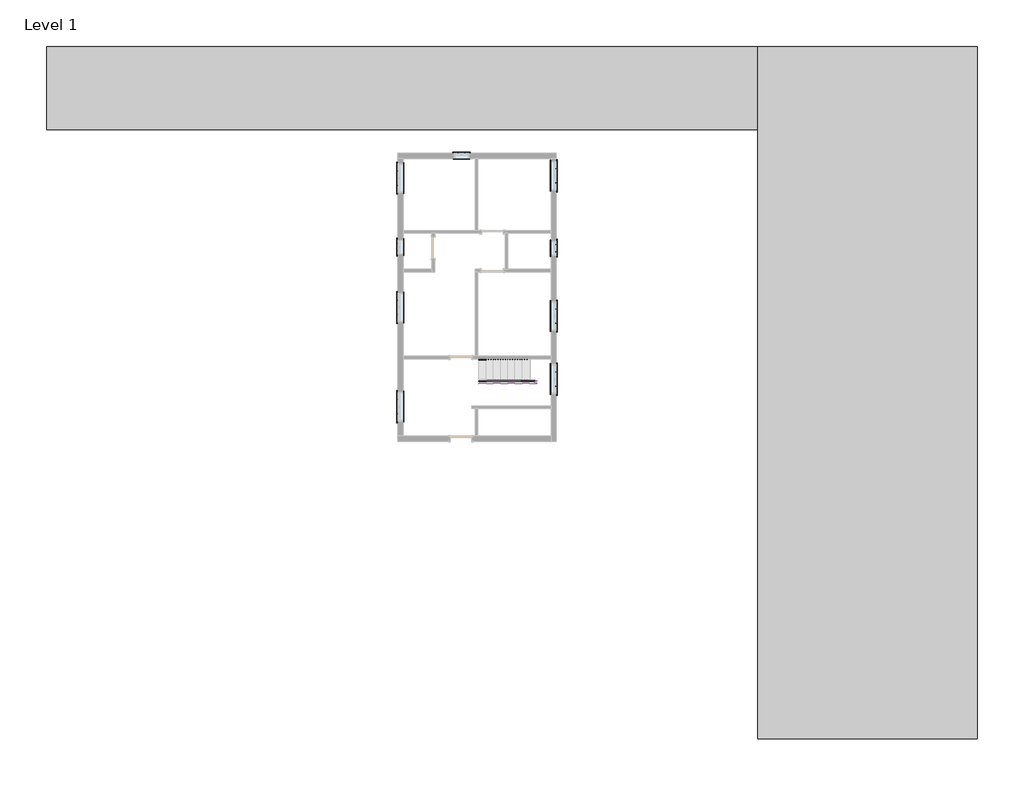
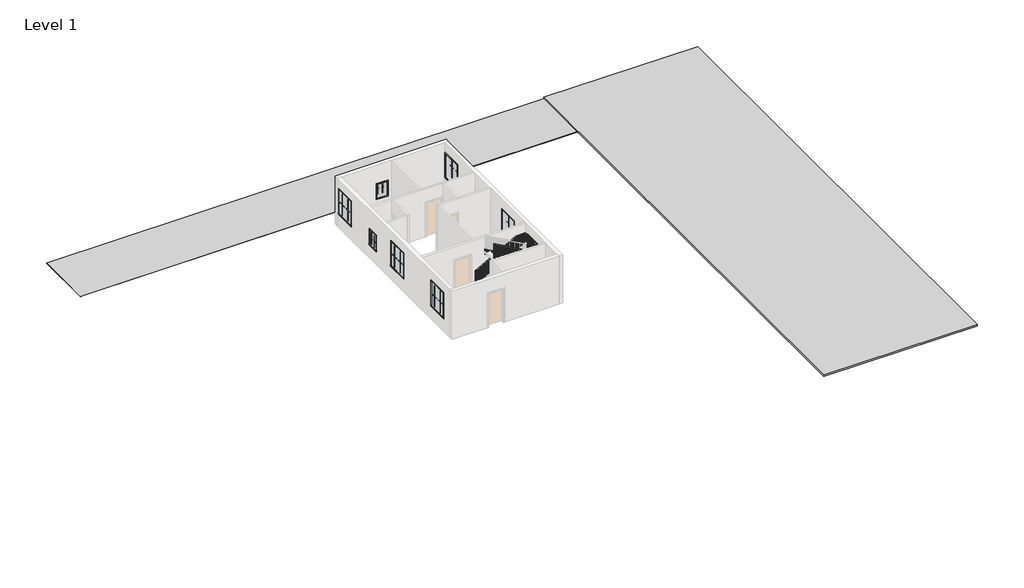
# One storey, part 2 of 2: 37 proxies, 3 members, 1 railing.
"""IFC4 building model written with IfcOpenShell, lengths in millimetres."""

from ifc_helpers import new_model, si_unit, frame, origin, place, context, project, spatial, polyline, outline, extrude, faceted_brep, transform, mapped, element, save
from components import generic_models_1_generic_models_1_c6e5ea94, muntin_pattern_2x2_muntin_pattern_2x2_6dad3731, muntin_pattern_2x2_muntin_pattern_2x2_a30a3345, muntin_pattern_2x2_muntin_pattern_2x2_53152e2c, muntin_pattern_2x2_muntin_pattern_2x2_e8f3e573, trim_window_exterior_flat_with_sill_92b9b949, trim_window_exterior_flat_with_sill_a665a915, trim_window_interior_flat_picture_frame_3bb882cf, trim_window_interior_flat_picture_frame_d485c387

model = new_model("IFC4")

# Units and contexts
model_context = context("Model", 3, world=origin())
ifc_project = project(units=[si_unit("LENGTHUNIT", "METRE", prefix="MILLI")], contexts=[model_context])

# Site, building, storey
site = spatial("IfcSite", under=ifc_project)
building = spatial("IfcBuilding", under=site)
storey = spatial("IfcBuildingStorey", under=building, Name="Level 1", Elevation=0.0)

# Proxies
placement = place(None, origin())
generic_models_1_generic_models_1_shape = generic_models_1_generic_models_1_c6e5ea94(model_context)
element("IfcBuildingElementProxy", 1, Name="Generic Models 1 : Generic Models 1", ObjectType="Generic Models 1 : Generic Models 1", at=placement, inside=storey, context=model_context, shape_type="MappedRepresentation", body=[
    mapped(generic_models_1_generic_models_1_shape, transform((0.0, 0.0, 0.0), x_axis=(1.0, 0.0, 0.0), y_axis=(0.0, 1.0, 0.0), z_axis=(0.0, 0.0, 1.0))),
])
muntin_pattern_2x2_muntin_pattern_2x2_shape = muntin_pattern_2x2_muntin_pattern_2x2_6dad3731(model_context)
element("IfcBuildingElementProxy", 2, Name="Muntin Pattern_2x2 : Muntin Pattern_2x2", ObjectType="Muntin Pattern_2x2 : Muntin Pattern_2x2", at=placement, inside=storey, context=model_context, shape_type="MappedRepresentation", body=[
    mapped(muntin_pattern_2x2_muntin_pattern_2x2_shape, transform((1279.525, 2947.4914062, 984.25), x_axis=(0.0, 1.0, 0.0), y_axis=(-1.0, 0.0, 0.0), z_axis=(0.0, 0.0, 1.0))),
])
element("IfcBuildingElementProxy", 3, Name="Muntin Pattern_2x2 : Muntin Pattern_2x2", ObjectType="Muntin Pattern_2x2 : Muntin Pattern_2x2", at=placement, inside=storey, context=model_context, shape_type="MappedRepresentation", body=[
    mapped(muntin_pattern_2x2_muntin_pattern_2x2_shape, transform((1279.525, 7141.6664062, 984.25), x_axis=(0.0, 1.0, 0.0), y_axis=(-1.0, 0.0, 0.0), z_axis=(0.0, 0.0, 1.0))),
])
element("IfcBuildingElementProxy", 4, Name="Muntin Pattern_2x2 : Muntin Pattern_2x2", ObjectType="Muntin Pattern_2x2 : Muntin Pattern_2x2", at=placement, inside=storey, context=model_context, shape_type="MappedRepresentation", body=[
    mapped(muntin_pattern_2x2_muntin_pattern_2x2_shape, transform((1279.525, 12605.8414062, 984.25), x_axis=(0.0, 1.0, 0.0), y_axis=(-1.0, 0.0, 0.0), z_axis=(0.0, 0.0, 1.0))),
])
element("IfcBuildingElementProxy", 5, Name="Muntin Pattern_2x2 : Muntin Pattern_2x2", ObjectType="Muntin Pattern_2x2 : Muntin Pattern_2x2", at=placement, inside=storey, context=model_context, shape_type="MappedRepresentation", body=[
    mapped(muntin_pattern_2x2_muntin_pattern_2x2_shape, transform((7966.075, 13308.0125, 984.25), x_axis=(0.0, -1.0, 0.0), y_axis=(1.0, 0.0, 0.0), z_axis=(0.0, 0.0, 1.0))),
])
element("IfcBuildingElementProxy", 6, Name="Muntin Pattern_2x2 : Muntin Pattern_2x2", ObjectType="Muntin Pattern_2x2 : Muntin Pattern_2x2", at=placement, inside=storey, context=model_context, shape_type="MappedRepresentation", body=[
    mapped(muntin_pattern_2x2_muntin_pattern_2x2_shape, transform((7966.075, 7377.1125, 984.25), x_axis=(0.0, -1.0, 0.0), y_axis=(1.0, 0.0, 0.0), z_axis=(0.0, 0.0, 1.0))),
])
element("IfcBuildingElementProxy", 7, Name="Muntin Pattern_2x2 : Muntin Pattern_2x2", ObjectType="Muntin Pattern_2x2 : Muntin Pattern_2x2", at=placement, inside=storey, context=model_context, shape_type="MappedRepresentation", body=[
    mapped(muntin_pattern_2x2_muntin_pattern_2x2_shape, transform((7966.075, 4716.4625, 984.25), x_axis=(0.0, -1.0, 0.0), y_axis=(1.0, 0.0, 0.0), z_axis=(0.0, 0.0, 1.0))),
])
muntin_pattern_2x2_muntin_pattern_2x2_2_shape = muntin_pattern_2x2_muntin_pattern_2x2_a30a3345(model_context)
element("IfcBuildingElementProxy", 8, Name="Muntin Pattern_2x2 : Muntin Pattern_2x2", ObjectType="Muntin Pattern_2x2 : Muntin Pattern_2x2", at=placement, inside=storey, context=model_context, shape_type="MappedRepresentation", body=[
    mapped(muntin_pattern_2x2_muntin_pattern_2x2_2_shape, transform((1279.525, 3553.9164063, 984.25), x_axis=(0.0, -1.0, 0.0), y_axis=(1.0, 0.0, 0.0), z_axis=(0.0, 0.0, 1.0))),
])
element("IfcBuildingElementProxy", 9, Name="Muntin Pattern_2x2 : Muntin Pattern_2x2", ObjectType="Muntin Pattern_2x2 : Muntin Pattern_2x2", at=placement, inside=storey, context=model_context, shape_type="MappedRepresentation", body=[
    mapped(muntin_pattern_2x2_muntin_pattern_2x2_2_shape, transform((1279.525, 7748.0914062, 984.25), x_axis=(0.0, -1.0, 0.0), y_axis=(1.0, 0.0, 0.0), z_axis=(0.0, 0.0, 1.0))),
])
element("IfcBuildingElementProxy", 10, Name="Muntin Pattern_2x2 : Muntin Pattern_2x2", ObjectType="Muntin Pattern_2x2 : Muntin Pattern_2x2", at=placement, inside=storey, context=model_context, shape_type="MappedRepresentation", body=[
    mapped(muntin_pattern_2x2_muntin_pattern_2x2_2_shape, transform((1279.525, 13212.2664062, 984.25), x_axis=(0.0, -1.0, 0.0), y_axis=(1.0, 0.0, 0.0), z_axis=(0.0, 0.0, 1.0))),
])
element("IfcBuildingElementProxy", 11, Name="Muntin Pattern_2x2 : Muntin Pattern_2x2", ObjectType="Muntin Pattern_2x2 : Muntin Pattern_2x2", at=placement, inside=storey, context=model_context, shape_type="MappedRepresentation", body=[
    mapped(muntin_pattern_2x2_muntin_pattern_2x2_2_shape, transform((7966.075, 12701.5875, 984.25), x_axis=(0.0, 1.0, 0.0), y_axis=(-1.0, 0.0, 0.0), z_axis=(0.0, 0.0, 1.0))),
])
element("IfcBuildingElementProxy", 12, Name="Muntin Pattern_2x2 : Muntin Pattern_2x2", ObjectType="Muntin Pattern_2x2 : Muntin Pattern_2x2", at=placement, inside=storey, context=model_context, shape_type="MappedRepresentation", body=[
    mapped(muntin_pattern_2x2_muntin_pattern_2x2_2_shape, transform((7966.075, 6770.6875, 984.25), x_axis=(0.0, 1.0, 0.0), y_axis=(-1.0, 0.0, 0.0), z_axis=(0.0, 0.0, 1.0))),
])
element("IfcBuildingElementProxy", 13, Name="Muntin Pattern_2x2 : Muntin Pattern_2x2", ObjectType="Muntin Pattern_2x2 : Muntin Pattern_2x2", at=placement, inside=storey, context=model_context, shape_type="MappedRepresentation", body=[
    mapped(muntin_pattern_2x2_muntin_pattern_2x2_2_shape, transform((7966.075, 4110.0375, 984.25), x_axis=(0.0, 1.0, 0.0), y_axis=(-1.0, 0.0, 0.0), z_axis=(0.0, 0.0, 1.0))),
])
muntin_pattern_2x2_muntin_pattern_2x2_3_shape = muntin_pattern_2x2_muntin_pattern_2x2_53152e2c(model_context)
element("IfcBuildingElementProxy", 14, Name="Muntin Pattern_2x2 : Muntin Pattern_2x2", ObjectType="Muntin Pattern_2x2 : Muntin Pattern_2x2", at=placement, inside=storey, context=model_context, shape_type="MappedRepresentation", body=[
    mapped(muntin_pattern_2x2_muntin_pattern_2x2_3_shape, transform((3811.5875, 13960.475, 984.25), x_axis=(1.0, 0.0, 0.0), y_axis=(0.0, 1.0, 0.0), z_axis=(0.0, 0.0, 1.0))),
])
element("IfcBuildingElementProxy", 15, Name="Muntin Pattern_2x2 : Muntin Pattern_2x2", ObjectType="Muntin Pattern_2x2 : Muntin Pattern_2x2", at=placement, inside=storey, context=model_context, shape_type="MappedRepresentation", body=[
    mapped(muntin_pattern_2x2_muntin_pattern_2x2_3_shape, transform((7966.075, 10101.2625, 984.25), x_axis=(0.0, -1.0, 0.0), y_axis=(1.0, 0.0, 0.0), z_axis=(0.0, 0.0, 1.0))),
])
element("IfcBuildingElementProxy", 16, Name="Muntin Pattern_2x2 : Muntin Pattern_2x2", ObjectType="Muntin Pattern_2x2 : Muntin Pattern_2x2", at=placement, inside=storey, context=model_context, shape_type="MappedRepresentation", body=[
    mapped(muntin_pattern_2x2_muntin_pattern_2x2_3_shape, transform((1279.525, 9843.5914062, 984.25), x_axis=(0.0, 1.0, 0.0), y_axis=(-1.0, 0.0, 0.0), z_axis=(0.0, 0.0, 1.0))),
])
muntin_pattern_2x2_muntin_pattern_2x2_4_shape = muntin_pattern_2x2_muntin_pattern_2x2_e8f3e573(model_context)
element("IfcBuildingElementProxy", 17, Name="Muntin Pattern_2x2 : Muntin Pattern_2x2", ObjectType="Muntin Pattern_2x2 : Muntin Pattern_2x2", at=placement, inside=storey, context=model_context, shape_type="MappedRepresentation", body=[
    mapped(muntin_pattern_2x2_muntin_pattern_2x2_4_shape, transform((4113.2125, 13960.475, 984.25), x_axis=(-1.0, 0.0, 0.0), y_axis=(0.0, -1.0, 0.0), z_axis=(0.0, 0.0, 1.0))),
])
element("IfcBuildingElementProxy", 18, Name="Muntin Pattern_2x2 : Muntin Pattern_2x2", ObjectType="Muntin Pattern_2x2 : Muntin Pattern_2x2", at=placement, inside=storey, context=model_context, shape_type="MappedRepresentation", body=[
    mapped(muntin_pattern_2x2_muntin_pattern_2x2_4_shape, transform((7966.075, 9799.6375, 984.25), x_axis=(0.0, 1.0, 0.0), y_axis=(-1.0, 0.0, 0.0), z_axis=(0.0, 0.0, 1.0))),
])
element("IfcBuildingElementProxy", 19, Name="Muntin Pattern_2x2 : Muntin Pattern_2x2", ObjectType="Muntin Pattern_2x2 : Muntin Pattern_2x2", at=placement, inside=storey, context=model_context, shape_type="MappedRepresentation", body=[
    mapped(muntin_pattern_2x2_muntin_pattern_2x2_4_shape, transform((1279.525, 10145.2164062, 984.25), x_axis=(0.0, -1.0, 0.0), y_axis=(1.0, 0.0, 0.0), z_axis=(0.0, 0.0, 1.0))),
])
trim_window_exterior_flat_with_sill_shape = trim_window_exterior_flat_with_sill_92b9b949(model_context)
element("IfcBuildingElementProxy", 20, Name="Trim-Window-Exterior-Flat : with Sill", ObjectType="Trim-Window-Exterior-Flat : with Sill", at=placement, inside=storey, context=model_context, shape_type="MappedRepresentation", body=[
    mapped(trim_window_exterior_flat_with_sill_shape, transform((1270.0, 3250.7039063, 2438.4), x_axis=(0.0, -1.0, 0.0), y_axis=(0.0, 0.0, 1.0), z_axis=(-1.0, 0.0, 0.0))),
])
element("IfcBuildingElementProxy", 21, Name="Trim-Window-Exterior-Flat : with Sill", ObjectType="Trim-Window-Exterior-Flat : with Sill", at=placement, inside=storey, context=model_context, shape_type="MappedRepresentation", body=[
    mapped(trim_window_exterior_flat_with_sill_shape, transform((1270.0, 7444.8789063, 2438.4), x_axis=(0.0, -1.0, 0.0), y_axis=(0.0, 0.0, 1.0), z_axis=(-1.0, 0.0, 0.0))),
])
element("IfcBuildingElementProxy", 22, Name="Trim-Window-Exterior-Flat : with Sill", ObjectType="Trim-Window-Exterior-Flat : with Sill", at=placement, inside=storey, context=model_context, shape_type="MappedRepresentation", body=[
    mapped(trim_window_exterior_flat_with_sill_shape, transform((1270.0, 12909.0539063, 2438.4), x_axis=(0.0, -1.0, 0.0), y_axis=(0.0, 0.0, 1.0), z_axis=(-1.0, 0.0, 0.0))),
])
element("IfcBuildingElementProxy", 23, Name="Trim-Window-Exterior-Flat : with Sill", ObjectType="Trim-Window-Exterior-Flat : with Sill", at=placement, inside=storey, context=model_context, shape_type="MappedRepresentation", body=[
    mapped(trim_window_exterior_flat_with_sill_shape, transform((7975.6, 13004.8, 2438.4), x_axis=(0.0, 1.0, 0.0), y_axis=(0.0, 0.0, 1.0), z_axis=(1.0, 0.0, 0.0))),
])
element("IfcBuildingElementProxy", 24, Name="Trim-Window-Exterior-Flat : with Sill", ObjectType="Trim-Window-Exterior-Flat : with Sill", at=placement, inside=storey, context=model_context, shape_type="MappedRepresentation", body=[
    mapped(trim_window_exterior_flat_with_sill_shape, transform((7975.6, 7073.9, 2438.4), x_axis=(0.0, 1.0, 0.0), y_axis=(0.0, 0.0, 1.0), z_axis=(1.0, 0.0, 0.0))),
])
element("IfcBuildingElementProxy", 25, Name="Trim-Window-Exterior-Flat : with Sill", ObjectType="Trim-Window-Exterior-Flat : with Sill", at=placement, inside=storey, context=model_context, shape_type="MappedRepresentation", body=[
    mapped(trim_window_exterior_flat_with_sill_shape, transform((7975.6, 4413.25, 2438.4), x_axis=(0.0, 1.0, 0.0), y_axis=(0.0, 0.0, 1.0), z_axis=(1.0, 0.0, 0.0))),
])
trim_window_exterior_flat_with_sill_2_shape = trim_window_exterior_flat_with_sill_a665a915(model_context)
element("IfcBuildingElementProxy", 26, Name="Trim-Window-Exterior-Flat : with Sill", ObjectType="Trim-Window-Exterior-Flat : with Sill", at=placement, inside=storey, context=model_context, shape_type="MappedRepresentation", body=[
    mapped(trim_window_exterior_flat_with_sill_2_shape, transform((3962.4, 13970.0, 1828.8), x_axis=(-1.0, 0.0, 0.0), y_axis=(0.0, 0.0, 1.0), z_axis=(0.0, 1.0, 0.0))),
])
element("IfcBuildingElementProxy", 27, Name="Trim-Window-Exterior-Flat : with Sill", ObjectType="Trim-Window-Exterior-Flat : with Sill", at=placement, inside=storey, context=model_context, shape_type="MappedRepresentation", body=[
    mapped(trim_window_exterior_flat_with_sill_2_shape, transform((7975.6, 9950.45, 1828.8), x_axis=(0.0, 1.0, 0.0), y_axis=(0.0, 0.0, 1.0), z_axis=(1.0, 0.0, 0.0))),
])
element("IfcBuildingElementProxy", 28, Name="Trim-Window-Exterior-Flat : with Sill", ObjectType="Trim-Window-Exterior-Flat : with Sill", at=placement, inside=storey, context=model_context, shape_type="MappedRepresentation", body=[
    mapped(trim_window_exterior_flat_with_sill_2_shape, transform((1270.0, 9994.4039062, 1828.8), x_axis=(0.0, -1.0, 0.0), y_axis=(0.0, 0.0, 1.0), z_axis=(-1.0, 0.0, 0.0))),
])
trim_window_interior_flat_picture_frame_shape = trim_window_interior_flat_picture_frame_3bb882cf(model_context)
element("IfcBuildingElementProxy", 29, Name="Trim-Window-Interior-Flat : Picture Frame", ObjectType="Trim-Window-Interior-Flat : Picture Frame", at=placement, inside=storey, context=model_context, shape_type="MappedRepresentation", body=[
    mapped(trim_window_interior_flat_picture_frame_shape, transform((1498.6, 3250.7039063, 2438.4), x_axis=(0.0, 1.0, 0.0), y_axis=(0.0, 0.0, 1.0), z_axis=(1.0, 0.0, 0.0))),
])
element("IfcBuildingElementProxy", 30, Name="Trim-Window-Interior-Flat : Picture Frame", ObjectType="Trim-Window-Interior-Flat : Picture Frame", at=placement, inside=storey, context=model_context, shape_type="MappedRepresentation", body=[
    mapped(trim_window_interior_flat_picture_frame_shape, transform((1498.6, 7444.8789062, 2438.4), x_axis=(0.0, 1.0, 0.0), y_axis=(0.0, 0.0, 1.0), z_axis=(1.0, 0.0, 0.0))),
])
element("IfcBuildingElementProxy", 31, Name="Trim-Window-Interior-Flat : Picture Frame", ObjectType="Trim-Window-Interior-Flat : Picture Frame", at=placement, inside=storey, context=model_context, shape_type="MappedRepresentation", body=[
    mapped(trim_window_interior_flat_picture_frame_shape, transform((1498.6, 12909.0539062, 2438.4), x_axis=(0.0, 1.0, 0.0), y_axis=(0.0, 0.0, 1.0), z_axis=(1.0, 0.0, 0.0))),
])
element("IfcBuildingElementProxy", 32, Name="Trim-Window-Interior-Flat : Picture Frame", ObjectType="Trim-Window-Interior-Flat : Picture Frame", at=placement, inside=storey, context=model_context, shape_type="MappedRepresentation", body=[
    mapped(trim_window_interior_flat_picture_frame_shape, transform((7747.0, 13004.8, 2438.4), x_axis=(0.0, -1.0, 0.0), y_axis=(0.0, 0.0, 1.0), z_axis=(-1.0, 0.0, 0.0))),
])
element("IfcBuildingElementProxy", 33, Name="Trim-Window-Interior-Flat : Picture Frame", ObjectType="Trim-Window-Interior-Flat : Picture Frame", at=placement, inside=storey, context=model_context, shape_type="MappedRepresentation", body=[
    mapped(trim_window_interior_flat_picture_frame_shape, transform((7747.0, 7073.9, 2438.4), x_axis=(0.0, -1.0, 0.0), y_axis=(0.0, 0.0, 1.0), z_axis=(-1.0, 0.0, 0.0))),
])
element("IfcBuildingElementProxy", 34, Name="Trim-Window-Interior-Flat : Picture Frame", ObjectType="Trim-Window-Interior-Flat : Picture Frame", at=placement, inside=storey, context=model_context, shape_type="MappedRepresentation", body=[
    mapped(trim_window_interior_flat_picture_frame_shape, transform((7747.0, 4413.25, 2438.4), x_axis=(0.0, -1.0, 0.0), y_axis=(0.0, 0.0, 1.0), z_axis=(-1.0, 0.0, 0.0))),
])
trim_window_interior_flat_picture_frame_2_shape = trim_window_interior_flat_picture_frame_d485c387(model_context)
element("IfcBuildingElementProxy", 35, Name="Trim-Window-Interior-Flat : Picture Frame", ObjectType="Trim-Window-Interior-Flat : Picture Frame", at=placement, inside=storey, context=model_context, shape_type="MappedRepresentation", body=[
    mapped(trim_window_interior_flat_picture_frame_2_shape, transform((3962.4, 13741.4, 1828.8), x_axis=(1.0, 0.0, 0.0), y_axis=(0.0, 0.0, 1.0), z_axis=(0.0, -1.0, 0.0))),
])
element("IfcBuildingElementProxy", 36, Name="Trim-Window-Interior-Flat : Picture Frame", ObjectType="Trim-Window-Interior-Flat : Picture Frame", at=placement, inside=storey, context=model_context, shape_type="MappedRepresentation", body=[
    mapped(trim_window_interior_flat_picture_frame_2_shape, transform((7747.0, 9950.45, 1828.8), x_axis=(0.0, -1.0, 0.0), y_axis=(0.0, 0.0, 1.0), z_axis=(-1.0, 0.0, 0.0))),
])
element("IfcBuildingElementProxy", 37, Name="Trim-Window-Interior-Flat : Picture Frame", ObjectType="Trim-Window-Interior-Flat : Picture Frame", at=placement, inside=storey, context=model_context, shape_type="MappedRepresentation", body=[
    mapped(trim_window_interior_flat_picture_frame_2_shape, transform((1498.6, 9994.4039062, 1828.8), x_axis=(0.0, 1.0, 0.0), y_axis=(0.0, 0.0, 1.0), z_axis=(1.0, 0.0, 0.0))),
])

# Members
element("IfcMember", 38, ObjectType="Stringer - 2\" Width", at=placement, inside=storey, context=model_context, shape_type="SweptSolid", body=[
    extrude(outline(polyline([(207.5983948, 4699.0), (0.0, 4699.0), (0.0, 4952.9445028), (1185.3641651, 7086.6), (1534.0428392, 7086.6), (207.5983948, 4699.0)])), frame((0.0, 4305.3, 0.0), z_axis=(0.0, 1.0, 0.0), x_axis=(0.0, 0.0, 1.0)), (0.0, 0.0, 1.0), 50.8),
])
element("IfcMember", 39, ObjectType="Stringer - 2\" Width", at=placement, inside=storey, context=model_context, shape_type="SweptSolid", body=[
    extrude(outline(polyline([(7086.6, 4356.1), (7137.4, 4356.1), (7137.4, 4254.5), (7086.6, 4254.5), (7086.6, 4356.1)])), frame((0.0, 0.0, 1295.4), z_axis=(0.0, 0.0, 1.0), x_axis=(1.0, 0.0, 0.0)), (0.0, 0.0, 1.0), 304.8),
])
element("IfcMember", 40, ObjectType="Stringer - 2\" Width", at=placement, inside=storey, context=model_context, shape_type="SweptSolid", body=[
    extrude(outline(polyline([(1382.9197207, 7137.4), (1731.5983948, 7137.4), (3086.2650614, 4699.0), (2737.5863873, 4699.0), (1382.9197207, 7137.4)])), frame((0.0, 4203.7, 0.0), z_axis=(0.0, 1.0, 0.0), x_axis=(0.0, 0.0, 1.0)), (0.0, 0.0, 1.0), 50.8),
])

# Railing
element("IfcRailing", 41, ObjectType="Handrail - Rectangular", at=placement, inside=storey, context=model_context, shape_type="SolidModel", body=[
    faceted_brep([(4699.0, 5270.5, 1083.7333333), (4699.0, 5270.5, 1025.620221), (4699.0, 5219.7, 1025.620221), (4699.0, 5219.7, 1083.7333333), (7137.4, 5270.5, 2438.4), (7150.5636022, 5270.5, 2387.6), (7150.5636022, 5219.7, 2387.6), (7137.4, 5219.7, 2438.4), (7747.0, 5270.5, 2438.4), (7747.0, 5270.5, 2387.6), (7696.2, 5219.7, 2387.6), (7696.2, 5219.7, 2438.4), (7747.0, 3289.3, 2438.4), (7747.0, 3289.3, 2387.6), (7696.2, 3340.1, 2387.6), (7696.2, 3340.1, 2438.4), (7442.2, 3289.3, 2438.4), (7429.0363978, 3289.3, 2387.6), (7429.0363978, 3340.1, 2387.6), (7442.2, 3340.1, 2438.4), (4699.0, 3289.3, 3962.4), (4699.0, 3340.1, 3962.4), (4699.0, 3340.1, 3904.2868876), (4699.0, 3289.3, 3904.2868876)], [[[0, 1, 2, 3]], [[1, 0, 4, 5]], [[2, 1, 5, 6]], [[3, 2, 6, 7]], [[0, 3, 7, 4]], [[5, 4, 8, 9]], [[6, 5, 9, 10]], [[7, 6, 10, 11]], [[4, 7, 11, 8]], [[9, 8, 12, 13]], [[10, 9, 13, 14]], [[11, 10, 14, 15]], [[8, 11, 15, 12]], [[13, 12, 16, 17]], [[14, 13, 17, 18]], [[15, 14, 18, 19]], [[12, 15, 19, 16]], [[20, 21, 22, 23]], [[17, 16, 20, 23]], [[18, 17, 23, 22]], [[19, 18, 22, 21]], [[16, 19, 21, 20]]]),
    extrude(outline(polyline([(3867.245221, 4765.675), (2878.6666667, 4765.675), (2878.6666667, 4784.725), (3856.6618876, 4784.725), (3867.245221, 4765.675)])), frame((0.0, 3305.175, 0.0), z_axis=(0.0, 1.0, 0.0), x_axis=(0.0, 0.0, 1.0)), (0.0, 0.0, 1.0), 19.05),
    extrude(outline(polyline([(3810.8007765, 4867.275), (2878.6666667, 4867.275), (2878.6666667, 4886.325), (3800.2174432, 4886.325), (3810.8007765, 4867.275)])), frame((0.0, 3305.175, 0.0), z_axis=(0.0, 1.0, 0.0), x_axis=(0.0, 0.0, 1.0)), (0.0, 0.0, 1.0), 19.05),
    extrude(outline(polyline([(3754.3563321, 4968.875), (2878.6666667, 4968.875), (2878.6666667, 4987.925), (3743.7729988, 4987.925), (3754.3563321, 4968.875)])), frame((0.0, 3305.175, 0.0), z_axis=(0.0, 1.0, 0.0), x_axis=(0.0, 0.0, 1.0)), (0.0, 0.0, 1.0), 19.05),
    extrude(outline(polyline([(3697.9118876, 5070.475), (2709.3333333, 5070.475), (2709.3333333, 5089.525), (3687.3285543, 5089.525), (3697.9118876, 5070.475)])), frame((0.0, 3305.175, 0.0), z_axis=(0.0, 1.0, 0.0), x_axis=(0.0, 0.0, 1.0)), (0.0, 0.0, 1.0), 19.05),
    extrude(outline(polyline([(3641.4674432, 5172.075), (2709.3333333, 5172.075), (2709.3333333, 5191.125), (3630.8841099, 5191.125), (3641.4674432, 5172.075)])), frame((0.0, 3305.175, 0.0), z_axis=(0.0, 1.0, 0.0), x_axis=(0.0, 0.0, 1.0)), (0.0, 0.0, 1.0), 19.05),
    extrude(outline(polyline([(3585.0229988, 5273.675), (2709.3333333, 5273.675), (2709.3333333, 5292.725), (3574.4396654, 5292.725), (3585.0229988, 5273.675)])), frame((0.0, 3305.175, 0.0), z_axis=(0.0, 1.0, 0.0), x_axis=(0.0, 0.0, 1.0)), (0.0, 0.0, 1.0), 19.05),
    extrude(outline(polyline([(3528.5785543, 5375.275), (2540.0, 5375.275), (2540.0, 5394.325), (3517.995221, 5394.325), (3528.5785543, 5375.275)])), frame((0.0, 3305.175, 0.0), z_axis=(0.0, 1.0, 0.0), x_axis=(0.0, 0.0, 1.0)), (0.0, 0.0, 1.0), 19.05),
    extrude(outline(polyline([(3472.1341099, 5476.875), (2540.0, 5476.875), (2540.0, 5495.925), (3461.5507765, 5495.925), (3472.1341099, 5476.875)])), frame((0.0, 3305.175, 0.0), z_axis=(0.0, 1.0, 0.0), x_axis=(0.0, 0.0, 1.0)), (0.0, 0.0, 1.0), 19.05),
    extrude(outline(polyline([(3415.6896654, 5578.475), (2540.0, 5578.475), (2540.0, 5597.525), (3405.1063321, 5597.525), (3415.6896654, 5578.475)])), frame((0.0, 3305.175, 0.0), z_axis=(0.0, 1.0, 0.0), x_axis=(0.0, 0.0, 1.0)), (0.0, 0.0, 1.0), 19.05),
    extrude(outline(polyline([(3359.245221, 5680.075), (2370.6666667, 5680.075), (2370.6666667, 5699.125), (3348.6618876, 5699.125), (3359.245221, 5680.075)])), frame((0.0, 3305.175, 0.0), z_axis=(0.0, 1.0, 0.0), x_axis=(0.0, 0.0, 1.0)), (0.0, 0.0, 1.0), 19.05),
    extrude(outline(polyline([(3302.8007765, 5781.675), (2370.6666667, 5781.675), (2370.6666667, 5800.725), (3292.2174432, 5800.725), (3302.8007765, 5781.675)])), frame((0.0, 3305.175, 0.0), z_axis=(0.0, 1.0, 0.0), x_axis=(0.0, 0.0, 1.0)), (0.0, 0.0, 1.0), 19.05),
    extrude(outline(polyline([(3246.3563321, 5883.275), (2370.6666667, 5883.275), (2370.6666667, 5902.325), (3235.7729988, 5902.325), (3246.3563321, 5883.275)])), frame((0.0, 3305.175, 0.0), z_axis=(0.0, 1.0, 0.0), x_axis=(0.0, 0.0, 1.0)), (0.0, 0.0, 1.0), 19.05),
    extrude(outline(polyline([(3189.9118876, 5984.875), (2201.3333333, 5984.875), (2201.3333333, 6003.925), (3179.3285543, 6003.925), (3189.9118876, 5984.875)])), frame((0.0, 3305.175, 0.0), z_axis=(0.0, 1.0, 0.0), x_axis=(0.0, 0.0, 1.0)), (0.0, 0.0, 1.0), 19.05),
    extrude(outline(polyline([(3133.4674432, 6086.475), (2201.3333333, 6086.475), (2201.3333333, 6105.525), (3122.8841099, 6105.525), (3133.4674432, 6086.475)])), frame((0.0, 3305.175, 0.0), z_axis=(0.0, 1.0, 0.0), x_axis=(0.0, 0.0, 1.0)), (0.0, 0.0, 1.0), 19.05),
    extrude(outline(polyline([(3077.0229988, 6188.075), (2201.3333333, 6188.075), (2201.3333333, 6207.125), (3066.4396654, 6207.125), (3077.0229988, 6188.075)])), frame((0.0, 3305.175, 0.0), z_axis=(0.0, 1.0, 0.0), x_axis=(0.0, 0.0, 1.0)), (0.0, 0.0, 1.0), 19.05),
    extrude(outline(polyline([(3020.5785543, 6289.675), (2032.0, 6289.675), (2032.0, 6308.725), (3009.995221, 6308.725), (3020.5785543, 6289.675)])), frame((0.0, 3305.175, 0.0), z_axis=(0.0, 1.0, 0.0), x_axis=(0.0, 0.0, 1.0)), (0.0, 0.0, 1.0), 19.05),
    extrude(outline(polyline([(2964.1341099, 6391.275), (2032.0, 6391.275), (2032.0, 6410.325), (2953.5507765, 6410.325), (2964.1341099, 6391.275)])), frame((0.0, 3305.175, 0.0), z_axis=(0.0, 1.0, 0.0), x_axis=(0.0, 0.0, 1.0)), (0.0, 0.0, 1.0), 19.05),
    extrude(outline(polyline([(2907.6896654, 6492.875), (2032.0, 6492.875), (2032.0, 6511.925), (2897.1063321, 6511.925), (2907.6896654, 6492.875)])), frame((0.0, 3305.175, 0.0), z_axis=(0.0, 1.0, 0.0), x_axis=(0.0, 0.0, 1.0)), (0.0, 0.0, 1.0), 19.05),
    extrude(outline(polyline([(2851.245221, 6594.475), (1862.6666667, 6594.475), (1862.6666667, 6613.525), (2840.6618876, 6613.525), (2851.245221, 6594.475)])), frame((0.0, 3305.175, 0.0), z_axis=(0.0, 1.0, 0.0), x_axis=(0.0, 0.0, 1.0)), (0.0, 0.0, 1.0), 19.05),
    extrude(outline(polyline([(2794.8007765, 6696.075), (1862.6666667, 6696.075), (1862.6666667, 6715.125), (2784.2174432, 6715.125), (2794.8007765, 6696.075)])), frame((0.0, 3305.175, 0.0), z_axis=(0.0, 1.0, 0.0), x_axis=(0.0, 0.0, 1.0)), (0.0, 0.0, 1.0), 19.05),
    extrude(outline(polyline([(2738.3563321, 6797.675), (1862.6666667, 6797.675), (1862.6666667, 6816.725), (2727.7729988, 6816.725), (2738.3563321, 6797.675)])), frame((0.0, 3305.175, 0.0), z_axis=(0.0, 1.0, 0.0), x_axis=(0.0, 0.0, 1.0)), (0.0, 0.0, 1.0), 19.05),
    extrude(outline(polyline([(2681.9118876, 6899.275), (1693.3333333, 6899.275), (1693.3333333, 6918.325), (2671.3285543, 6918.325), (2681.9118876, 6899.275)])), frame((0.0, 3305.175, 0.0), z_axis=(0.0, 1.0, 0.0), x_axis=(0.0, 0.0, 1.0)), (0.0, 0.0, 1.0), 19.05),
    extrude(outline(polyline([(2625.4674432, 7000.875), (1693.3333333, 7000.875), (1693.3333333, 7019.925), (2614.8841099, 7019.925), (2625.4674432, 7000.875)])), frame((0.0, 3305.175, 0.0), z_axis=(0.0, 1.0, 0.0), x_axis=(0.0, 0.0, 1.0)), (0.0, 0.0, 1.0), 19.05),
    extrude(outline(polyline([(2569.0229988, 7102.475), (1693.3333333, 7102.475), (1693.3333333, 7121.525), (2558.4396654, 7121.525), (2569.0229988, 7102.475)])), frame((0.0, 3305.175, 0.0), z_axis=(0.0, 1.0, 0.0), x_axis=(0.0, 0.0, 1.0)), (0.0, 0.0, 1.0), 19.05),
    extrude(outline(polyline([(2512.5785543, 7204.075), (1524.0, 7204.075), (1524.0, 7223.125), (2501.995221, 7223.125), (2512.5785543, 7204.075)])), frame((0.0, 3305.175, 0.0), z_axis=(0.0, 1.0, 0.0), x_axis=(0.0, 0.0, 1.0)), (0.0, 0.0, 1.0), 19.05),
    extrude(outline(polyline([(2456.1341099, 7305.675), (1524.0, 7305.675), (1524.0, 7324.725), (2445.5507765, 7324.725), (2456.1341099, 7305.675)])), frame((0.0, 3305.175, 0.0), z_axis=(0.0, 1.0, 0.0), x_axis=(0.0, 0.0, 1.0)), (0.0, 0.0, 1.0), 19.05),
    extrude(outline(polyline([(2399.6896654, 7407.275), (1524.0, 7407.275), (1524.0, 7426.325), (2389.1063321, 7426.325), (2399.6896654, 7407.275)])), frame((0.0, 3305.175, 0.0), z_axis=(0.0, 1.0, 0.0), x_axis=(0.0, 0.0, 1.0)), (0.0, 0.0, 1.0), 19.05),
    extrude(outline(polyline([(7527.925, 3305.175), (7508.875, 3305.175), (7508.875, 3324.225), (7527.925, 3324.225), (7527.925, 3305.175)])), frame((0.0, 0.0, 1524.0), z_axis=(0.0, 0.0, 1.0), x_axis=(1.0, 0.0, 0.0)), (0.0, 0.0, 1.0), 863.6),
    extrude(outline(polyline([(7629.525, 3305.175), (7610.475, 3305.175), (7610.475, 3324.225), (7629.525, 3324.225), (7629.525, 3305.175)])), frame((0.0, 0.0, 1524.0), z_axis=(0.0, 0.0, 1.0), x_axis=(1.0, 0.0, 0.0)), (0.0, 0.0, 1.0), 863.6),
    extrude(outline(polyline([(7731.125, 3425.825), (7731.125, 3406.775), (7712.075, 3406.775), (7712.075, 3425.825), (7731.125, 3425.825)])), frame((0.0, 0.0, 1524.0), z_axis=(0.0, 0.0, 1.0), x_axis=(1.0, 0.0, 0.0)), (0.0, 0.0, 1.0), 863.6),
    extrude(outline(polyline([(7731.125, 3527.425), (7731.125, 3508.375), (7712.075, 3508.375), (7712.075, 3527.425), (7731.125, 3527.425)])), frame((0.0, 0.0, 1524.0), z_axis=(0.0, 0.0, 1.0), x_axis=(1.0, 0.0, 0.0)), (0.0, 0.0, 1.0), 863.6),
    extrude(outline(polyline([(7731.125, 3629.025), (7731.125, 3609.975), (7712.075, 3609.975), (7712.075, 3629.025), (7731.125, 3629.025)])), frame((0.0, 0.0, 1524.0), z_axis=(0.0, 0.0, 1.0), x_axis=(1.0, 0.0, 0.0)), (0.0, 0.0, 1.0), 863.6),
    extrude(outline(polyline([(7731.125, 3730.625), (7731.125, 3711.575), (7712.075, 3711.575), (7712.075, 3730.625), (7731.125, 3730.625)])), frame((0.0, 0.0, 1524.0), z_axis=(0.0, 0.0, 1.0), x_axis=(1.0, 0.0, 0.0)), (0.0, 0.0, 1.0), 863.6),
    extrude(outline(polyline([(7731.125, 3832.225), (7731.125, 3813.175), (7712.075, 3813.175), (7712.075, 3832.225), (7731.125, 3832.225)])), frame((0.0, 0.0, 1524.0), z_axis=(0.0, 0.0, 1.0), x_axis=(1.0, 0.0, 0.0)), (0.0, 0.0, 1.0), 863.6),
    extrude(outline(polyline([(7731.125, 3933.825), (7731.125, 3914.775), (7712.075, 3914.775), (7712.075, 3933.825), (7731.125, 3933.825)])), frame((0.0, 0.0, 1524.0), z_axis=(0.0, 0.0, 1.0), x_axis=(1.0, 0.0, 0.0)), (0.0, 0.0, 1.0), 863.6),
    extrude(outline(polyline([(7731.125, 4035.425), (7731.125, 4016.375), (7712.075, 4016.375), (7712.075, 4035.425), (7731.125, 4035.425)])), frame((0.0, 0.0, 1524.0), z_axis=(0.0, 0.0, 1.0), x_axis=(1.0, 0.0, 0.0)), (0.0, 0.0, 1.0), 863.6),
    extrude(outline(polyline([(7731.125, 4137.025), (7731.125, 4117.975), (7712.075, 4117.975), (7712.075, 4137.025), (7731.125, 4137.025)])), frame((0.0, 0.0, 1524.0), z_axis=(0.0, 0.0, 1.0), x_axis=(1.0, 0.0, 0.0)), (0.0, 0.0, 1.0), 863.6),
    extrude(outline(polyline([(7731.125, 4238.625), (7731.125, 4219.575), (7712.075, 4219.575), (7712.075, 4238.625), (7731.125, 4238.625)])), frame((0.0, 0.0, 1524.0), z_axis=(0.0, 0.0, 1.0), x_axis=(1.0, 0.0, 0.0)), (0.0, 0.0, 1.0), 863.6),
    extrude(outline(polyline([(7731.125, 4340.225), (7731.125, 4321.175), (7712.075, 4321.175), (7712.075, 4340.225), (7731.125, 4340.225)])), frame((0.0, 0.0, 1524.0), z_axis=(0.0, 0.0, 1.0), x_axis=(1.0, 0.0, 0.0)), (0.0, 0.0, 1.0), 863.6),
    extrude(outline(polyline([(7731.125, 4441.825), (7731.125, 4422.775), (7712.075, 4422.775), (7712.075, 4441.825), (7731.125, 4441.825)])), frame((0.0, 0.0, 1524.0), z_axis=(0.0, 0.0, 1.0), x_axis=(1.0, 0.0, 0.0)), (0.0, 0.0, 1.0), 863.6),
    extrude(outline(polyline([(7731.125, 4543.425), (7731.125, 4524.375), (7712.075, 4524.375), (7712.075, 4543.425), (7731.125, 4543.425)])), frame((0.0, 0.0, 1524.0), z_axis=(0.0, 0.0, 1.0), x_axis=(1.0, 0.0, 0.0)), (0.0, 0.0, 1.0), 863.6),
    extrude(outline(polyline([(7731.125, 4645.025), (7731.125, 4625.975), (7712.075, 4625.975), (7712.075, 4645.025), (7731.125, 4645.025)])), frame((0.0, 0.0, 1524.0), z_axis=(0.0, 0.0, 1.0), x_axis=(1.0, 0.0, 0.0)), (0.0, 0.0, 1.0), 863.6),
    extrude(outline(polyline([(7731.125, 4746.625), (7731.125, 4727.575), (7712.075, 4727.575), (7712.075, 4746.625), (7731.125, 4746.625)])), frame((0.0, 0.0, 1524.0), z_axis=(0.0, 0.0, 1.0), x_axis=(1.0, 0.0, 0.0)), (0.0, 0.0, 1.0), 863.6),
    extrude(outline(polyline([(7731.125, 4848.225), (7731.125, 4829.175), (7712.075, 4829.175), (7712.075, 4848.225), (7731.125, 4848.225)])), frame((0.0, 0.0, 1524.0), z_axis=(0.0, 0.0, 1.0), x_axis=(1.0, 0.0, 0.0)), (0.0, 0.0, 1.0), 863.6),
    extrude(outline(polyline([(7731.125, 4949.825), (7731.125, 4930.775), (7712.075, 4930.775), (7712.075, 4949.825), (7731.125, 4949.825)])), frame((0.0, 0.0, 1524.0), z_axis=(0.0, 0.0, 1.0), x_axis=(1.0, 0.0, 0.0)), (0.0, 0.0, 1.0), 863.6),
    extrude(outline(polyline([(7731.125, 5051.425), (7731.125, 5032.375), (7712.075, 5032.375), (7712.075, 5051.425), (7731.125, 5051.425)])), frame((0.0, 0.0, 1524.0), z_axis=(0.0, 0.0, 1.0), x_axis=(1.0, 0.0, 0.0)), (0.0, 0.0, 1.0), 863.6),
    extrude(outline(polyline([(7731.125, 5153.025), (7731.125, 5133.975), (7712.075, 5133.975), (7712.075, 5153.025), (7731.125, 5153.025)])), frame((0.0, 0.0, 1524.0), z_axis=(0.0, 0.0, 1.0), x_axis=(1.0, 0.0, 0.0)), (0.0, 0.0, 1.0), 863.6),
    extrude(outline(polyline([(7635.875, 5254.625), (7654.925, 5254.625), (7654.925, 5235.575), (7635.875, 5235.575), (7635.875, 5254.625)])), frame((0.0, 0.0, 1524.0), z_axis=(0.0, 0.0, 1.0), x_axis=(1.0, 0.0, 0.0)), (0.0, 0.0, 1.0), 863.6),
    extrude(outline(polyline([(7534.275, 5254.625), (7553.325, 5254.625), (7553.325, 5235.575), (7534.275, 5235.575), (7534.275, 5254.625)])), frame((0.0, 0.0, 1524.0), z_axis=(0.0, 0.0, 1.0), x_axis=(1.0, 0.0, 0.0)), (0.0, 0.0, 1.0), 863.6),
    extrude(outline(polyline([(7432.675, 5254.625), (7451.725, 5254.625), (7451.725, 5235.575), (7432.675, 5235.575), (7432.675, 5254.625)])), frame((0.0, 0.0, 1524.0), z_axis=(0.0, 0.0, 1.0), x_axis=(1.0, 0.0, 0.0)), (0.0, 0.0, 1.0), 863.6),
    extrude(outline(polyline([(7331.075, 5254.625), (7350.125, 5254.625), (7350.125, 5235.575), (7331.075, 5235.575), (7331.075, 5254.625)])), frame((0.0, 0.0, 1524.0), z_axis=(0.0, 0.0, 1.0), x_axis=(1.0, 0.0, 0.0)), (0.0, 0.0, 1.0), 863.6),
    extrude(outline(polyline([(7229.475, 5254.625), (7248.525, 5254.625), (7248.525, 5235.575), (7229.475, 5235.575), (7229.475, 5254.625)])), frame((0.0, 0.0, 1524.0), z_axis=(0.0, 0.0, 1.0), x_axis=(1.0, 0.0, 0.0)), (0.0, 0.0, 1.0), 863.6),
    extrude(outline(polyline([(2374.995221, 7127.875), (1524.0, 7127.875), (1524.0, 7146.925), (2385.5785543, 7146.925), (2374.995221, 7127.875)])), frame((0.0, 5235.575, 0.0), z_axis=(0.0, 1.0, 0.0), x_axis=(0.0, 0.0, 1.0)), (0.0, 0.0, 1.0), 19.05),
    extrude(outline(polyline([(2318.5507765, 7026.275), (1354.6666667, 7026.275), (1354.6666667, 7045.325), (2329.1341099, 7045.325), (2318.5507765, 7026.275)])), frame((0.0, 5235.575, 0.0), z_axis=(0.0, 1.0, 0.0), x_axis=(0.0, 0.0, 1.0)), (0.0, 0.0, 1.0), 19.05),
    extrude(outline(polyline([(2262.1063321, 6924.675), (1354.6666667, 6924.675), (1354.6666667, 6943.725), (2272.6896654, 6943.725), (2262.1063321, 6924.675)])), frame((0.0, 5235.575, 0.0), z_axis=(0.0, 1.0, 0.0), x_axis=(0.0, 0.0, 1.0)), (0.0, 0.0, 1.0), 19.05),
    extrude(outline(polyline([(2205.6618876, 6823.075), (1354.6666667, 6823.075), (1354.6666667, 6842.125), (2216.245221, 6842.125), (2205.6618876, 6823.075)])), frame((0.0, 5235.575, 0.0), z_axis=(0.0, 1.0, 0.0), x_axis=(0.0, 0.0, 1.0)), (0.0, 0.0, 1.0), 19.05),
    extrude(outline(polyline([(2149.2174432, 6721.475), (1185.3333333, 6721.475), (1185.3333333, 6740.525), (2159.8007765, 6740.525), (2149.2174432, 6721.475)])), frame((0.0, 5235.575, 0.0), z_axis=(0.0, 1.0, 0.0), x_axis=(0.0, 0.0, 1.0)), (0.0, 0.0, 1.0), 19.05),
    extrude(outline(polyline([(2092.7729988, 6619.875), (1185.3333333, 6619.875), (1185.3333333, 6638.925), (2103.3563321, 6638.925), (2092.7729988, 6619.875)])), frame((0.0, 5235.575, 0.0), z_axis=(0.0, 1.0, 0.0), x_axis=(0.0, 0.0, 1.0)), (0.0, 0.0, 1.0), 19.05),
    extrude(outline(polyline([(2036.3285543, 6518.275), (1185.3333333, 6518.275), (1185.3333333, 6537.325), (2046.9118876, 6537.325), (2036.3285543, 6518.275)])), frame((0.0, 5235.575, 0.0), z_axis=(0.0, 1.0, 0.0), x_axis=(0.0, 0.0, 1.0)), (0.0, 0.0, 1.0), 19.05),
    extrude(outline(polyline([(1979.8841099, 6416.675), (1016.0, 6416.675), (1016.0, 6435.725), (1990.4674432, 6435.725), (1979.8841099, 6416.675)])), frame((0.0, 5235.575, 0.0), z_axis=(0.0, 1.0, 0.0), x_axis=(0.0, 0.0, 1.0)), (0.0, 0.0, 1.0), 19.05),
    extrude(outline(polyline([(1923.4396654, 6315.075), (1016.0, 6315.075), (1016.0, 6334.125), (1934.0229988, 6334.125), (1923.4396654, 6315.075)])), frame((0.0, 5235.575, 0.0), z_axis=(0.0, 1.0, 0.0), x_axis=(0.0, 0.0, 1.0)), (0.0, 0.0, 1.0), 19.05),
    extrude(outline(polyline([(1866.995221, 6213.475), (1016.0, 6213.475), (1016.0, 6232.525), (1877.5785543, 6232.525), (1866.995221, 6213.475)])), frame((0.0, 5235.575, 0.0), z_axis=(0.0, 1.0, 0.0), x_axis=(0.0, 0.0, 1.0)), (0.0, 0.0, 1.0), 19.05),
    extrude(outline(polyline([(1810.5507765, 6111.875), (846.6666667, 6111.875), (846.6666667, 6130.925), (1821.1341099, 6130.925), (1810.5507765, 6111.875)])), frame((0.0, 5235.575, 0.0), z_axis=(0.0, 1.0, 0.0), x_axis=(0.0, 0.0, 1.0)), (0.0, 0.0, 1.0), 19.05),
    extrude(outline(polyline([(1754.1063321, 6010.275), (846.6666667, 6010.275), (846.6666667, 6029.325), (1764.6896654, 6029.325), (1754.1063321, 6010.275)])), frame((0.0, 5235.575, 0.0), z_axis=(0.0, 1.0, 0.0), x_axis=(0.0, 0.0, 1.0)), (0.0, 0.0, 1.0), 19.05),
    extrude(outline(polyline([(1697.6618876, 5908.675), (846.6666667, 5908.675), (846.6666667, 5927.725), (1708.245221, 5927.725), (1697.6618876, 5908.675)])), frame((0.0, 5235.575, 0.0), z_axis=(0.0, 1.0, 0.0), x_axis=(0.0, 0.0, 1.0)), (0.0, 0.0, 1.0), 19.05),
    extrude(outline(polyline([(1641.2174432, 5807.075), (677.3333333, 5807.075), (677.3333333, 5826.125), (1651.8007765, 5826.125), (1641.2174432, 5807.075)])), frame((0.0, 5235.575, 0.0), z_axis=(0.0, 1.0, 0.0), x_axis=(0.0, 0.0, 1.0)), (0.0, 0.0, 1.0), 19.05),
    extrude(outline(polyline([(1584.7729988, 5705.475), (677.3333333, 5705.475), (677.3333333, 5724.525), (1595.3563321, 5724.525), (1584.7729988, 5705.475)])), frame((0.0, 5235.575, 0.0), z_axis=(0.0, 1.0, 0.0), x_axis=(0.0, 0.0, 1.0)), (0.0, 0.0, 1.0), 19.05),
    extrude(outline(polyline([(1528.3285543, 5603.875), (677.3333333, 5603.875), (677.3333333, 5622.925), (1538.9118876, 5622.925), (1528.3285543, 5603.875)])), frame((0.0, 5235.575, 0.0), z_axis=(0.0, 1.0, 0.0), x_axis=(0.0, 0.0, 1.0)), (0.0, 0.0, 1.0), 19.05),
    extrude(outline(polyline([(1471.8841099, 5502.275), (508.0, 5502.275), (508.0, 5521.325), (1482.4674432, 5521.325), (1471.8841099, 5502.275)])), frame((0.0, 5235.575, 0.0), z_axis=(0.0, 1.0, 0.0), x_axis=(0.0, 0.0, 1.0)), (0.0, 0.0, 1.0), 19.05),
    extrude(outline(polyline([(1415.4396654, 5400.675), (508.0, 5400.675), (508.0, 5419.725), (1426.0229988, 5419.725), (1415.4396654, 5400.675)])), frame((0.0, 5235.575, 0.0), z_axis=(0.0, 1.0, 0.0), x_axis=(0.0, 0.0, 1.0)), (0.0, 0.0, 1.0), 19.05),
    extrude(outline(polyline([(1358.995221, 5299.075), (508.0, 5299.075), (508.0, 5318.125), (1369.5785543, 5318.125), (1358.995221, 5299.075)])), frame((0.0, 5235.575, 0.0), z_axis=(0.0, 1.0, 0.0), x_axis=(0.0, 0.0, 1.0)), (0.0, 0.0, 1.0), 19.05),
    extrude(outline(polyline([(1302.5507765, 5197.475), (338.6666667, 5197.475), (338.6666667, 5216.525), (1313.1341099, 5216.525), (1302.5507765, 5197.475)])), frame((0.0, 5235.575, 0.0), z_axis=(0.0, 1.0, 0.0), x_axis=(0.0, 0.0, 1.0)), (0.0, 0.0, 1.0), 19.05),
    extrude(outline(polyline([(1246.1063321, 5095.875), (338.6666667, 5095.875), (338.6666667, 5114.925), (1256.6896654, 5114.925), (1246.1063321, 5095.875)])), frame((0.0, 5235.575, 0.0), z_axis=(0.0, 1.0, 0.0), x_axis=(0.0, 0.0, 1.0)), (0.0, 0.0, 1.0), 19.05),
    extrude(outline(polyline([(1189.6618876, 4994.275), (338.6666667, 4994.275), (338.6666667, 5013.325), (1200.245221, 5013.325), (1189.6618876, 4994.275)])), frame((0.0, 5235.575, 0.0), z_axis=(0.0, 1.0, 0.0), x_axis=(0.0, 0.0, 1.0)), (0.0, 0.0, 1.0), 19.05),
    extrude(outline(polyline([(1133.2174432, 4892.675), (169.3333333, 4892.675), (169.3333333, 4911.725), (1143.8007765, 4911.725), (1133.2174432, 4892.675)])), frame((0.0, 5235.575, 0.0), z_axis=(0.0, 1.0, 0.0), x_axis=(0.0, 0.0, 1.0)), (0.0, 0.0, 1.0), 19.05),
    extrude(outline(polyline([(1076.7729988, 4791.075), (169.3333333, 4791.075), (169.3333333, 4810.125), (1087.3563321, 4810.125), (1076.7729988, 4791.075)])), frame((0.0, 5235.575, 0.0), z_axis=(0.0, 1.0, 0.0), x_axis=(0.0, 0.0, 1.0)), (0.0, 0.0, 1.0), 19.05),
    extrude(outline(polyline([(7731.125, 3324.225), (7731.125, 3305.175), (7712.075, 3305.175), (7712.075, 3324.225), (7731.125, 3324.225)])), frame((0.0, 0.0, 1524.0), z_axis=(0.0, 0.0, 1.0), x_axis=(1.0, 0.0, 0.0)), (0.0, 0.0, 1.0), 863.6),
    extrude(outline(polyline([(7712.075, 5254.625), (7731.125, 5254.625), (7731.125, 5235.575), (7712.075, 5235.575), (7712.075, 5254.625)])), frame((0.0, 0.0, 1524.0), z_axis=(0.0, 0.0, 1.0), x_axis=(1.0, 0.0, 0.0)), (0.0, 0.0, 1.0), 863.6),
    extrude(outline(polyline([(3904.2868876, 4699.0), (2878.6666667, 4699.0), (2878.6666667, 4718.05), (3893.7035543, 4718.05), (3904.2868876, 4699.0)])), frame((0.0, 3305.175, 0.0), z_axis=(0.0, 1.0, 0.0), x_axis=(0.0, 0.0, 1.0)), (0.0, 0.0, 1.0), 19.05),
    extrude(outline(polyline([(1025.620221, 4699.0), (169.3333333, 4699.0), (169.3333333, 4718.05), (1036.2035543, 4718.05), (1025.620221, 4699.0)])), frame((0.0, 5235.575, 0.0), z_axis=(0.0, 1.0, 0.0), x_axis=(0.0, 0.0, 1.0)), (0.0, 0.0, 1.0), 19.05),
])

save(model, "model.ifc")

# Revit data of these elements
# Type "Muntin Pattern_2x2 : Muntin Pattern_2x2"
#   Width [instance default] = 4' - 0"
#   Thickness = 0' - 0 1/2"
#   Height [instance default] = 4' - 0"
#   Distance = 0' - 0 3/4"
#   Interior Material [instance default] = none
#   Exterior Material [instance default] = none
#   Default Elevation = 0
# Type "Trim-Window-Exterior-Flat : with Sill"
#   Trim Width = 0' - 2 1/4"
#   Trim Thickness_Picture Frame = 0' - 1 1/4"
#   Trim Thickness_with Sill = 0' - 0 3/4"
#   Sill Thickness = 0' - 1 1/4"
#   Opening Width [instance default] = 2' - 0"
#   Opening Height [instance default] = 3' - 0"
#   Default Elevation = 4' - 0"
#   Sill = yes
#   Picture Frame = no
#   Trim Material [instance default] = none
# Type "Trim-Window-Interior-Flat : Picture Frame"
#   Trim Thickness_Picture Frame = 0' - 1 1/4"
#   Trim Width = 0' - 2 1/4"
#   Trim Thickness_with Sill = 0' - 0 3/4"
#   Sill Thickness = 0' - 1 1/4"
#   Opening Width [instance default] = 2' - 0"
#   Opening Height [instance default] = 3' - 0"
#   Default Elevation = 4' - 0"
#   Sill = no
#   Picture Frame = yes
#   Trim Material [instance default] = none
# Type "Handrail - Rectangular"
#   Assembly Code = "C2010400"
#   built-in parameter 1008612 = 0.0416667 (stored number, unit not read)
#   built-in parameter 1008611 = 0.0416667 (stored number, unit not read)
#   built-in parameter 1008609 = 0.333333 (stored number, unit not read)
#   built-in parameter 1008604 = 0.166667 (stored number, unit not read)
#   built-in parameter 1008603 = 0.166667 (stored number, unit not read)
#   Railing Height = 3' - 0"
#   built-in parameter 1008630 = 2
#   built-in parameter 1008610 = 2
#   built-in parameter 1008618 = Baluster - Square : 3/4"
# Element 1 (IfcBuildingElementProxy, "Generic Models 1 : Generic Models 1")
#   Phase Created = New Construction
# Elements 2, 3, 4, 5, 6, 7, 8, 9, 10, 11, 12, 13 (IfcBuildingElementProxy, "Muntin Pattern_2x2 : Muntin Pattern_2x2")
#   Width = 1' - 6 5/8"
#   Height = 4' - 6 1/2"
#   Interior Material = Wood - Stained
#   Exterior Material = Clad - White
#   Phase Created = New Construction
#   Materials on its faces: "Clad - White", "Wood - Stained"
# Elements 14, 15, 16, 17, 18, 19 (IfcBuildingElementProxy, "Muntin Pattern_2x2 : Muntin Pattern_2x2")
#   Width = 0' - 6 5/8"
#   Height = 2' - 6 1/2"
#   Interior Material = Wood - Stained
#   Exterior Material = Clad - White
#   Phase Created = New Construction
#   Materials on its faces: "Clad - White", "Wood - Stained"
# Elements 20, 21, 22, 23, 24, 25 (IfcBuildingElementProxy, "Trim-Window-Exterior-Flat : with Sill")
#   Opening Width = 4' - 0"
#   Opening Height = 5' - 0"
#   Trim Material = Clad - White
#   Phase Created = New Construction
#   Materials on its faces: "Clad - White"
# Elements 26, 27, 28 (IfcBuildingElementProxy, "Trim-Window-Exterior-Flat : with Sill")
#   Opening Width = 2' - 0"
#   Opening Height = 3' - 0"
#   Trim Material = Clad - White
#   Phase Created = New Construction
#   Materials on its faces: "Clad - White"
# Elements 29, 30, 31, 32, 33, 34 (IfcBuildingElementProxy, "Trim-Window-Interior-Flat : Picture Frame")
#   Opening Width = 4' - 0"
#   Opening Height = 5' - 0"
#   Trim Material = Wood - Stained
#   Phase Created = New Construction
#   Materials on its faces: "Wood - Stained"
# Elements 35, 36, 37 (IfcBuildingElementProxy, "Trim-Window-Interior-Flat : Picture Frame")
#   Opening Width = 2' - 0"
#   Opening Height = 3' - 0"
#   Trim Material = Wood - Stained
#   Phase Created = New Construction
#   Materials on its faces: "Wood - Stained"
# Elements 38, 39, 40 (IfcMember, "Stringer - 2\" Width")
#   Phase Created = New Construction
# Element 41 (IfcRailing, "Handrail - Rectangular")
#   Phase Created = New Construction
# Materials
#   "Clad - White": class "Wood", colour RGB 242 242 238, transparency 0, Cost = 0
#   "Wood - Stained": class "Wood", colour RGB 224 178 126, transparency 0, Cost = 0
